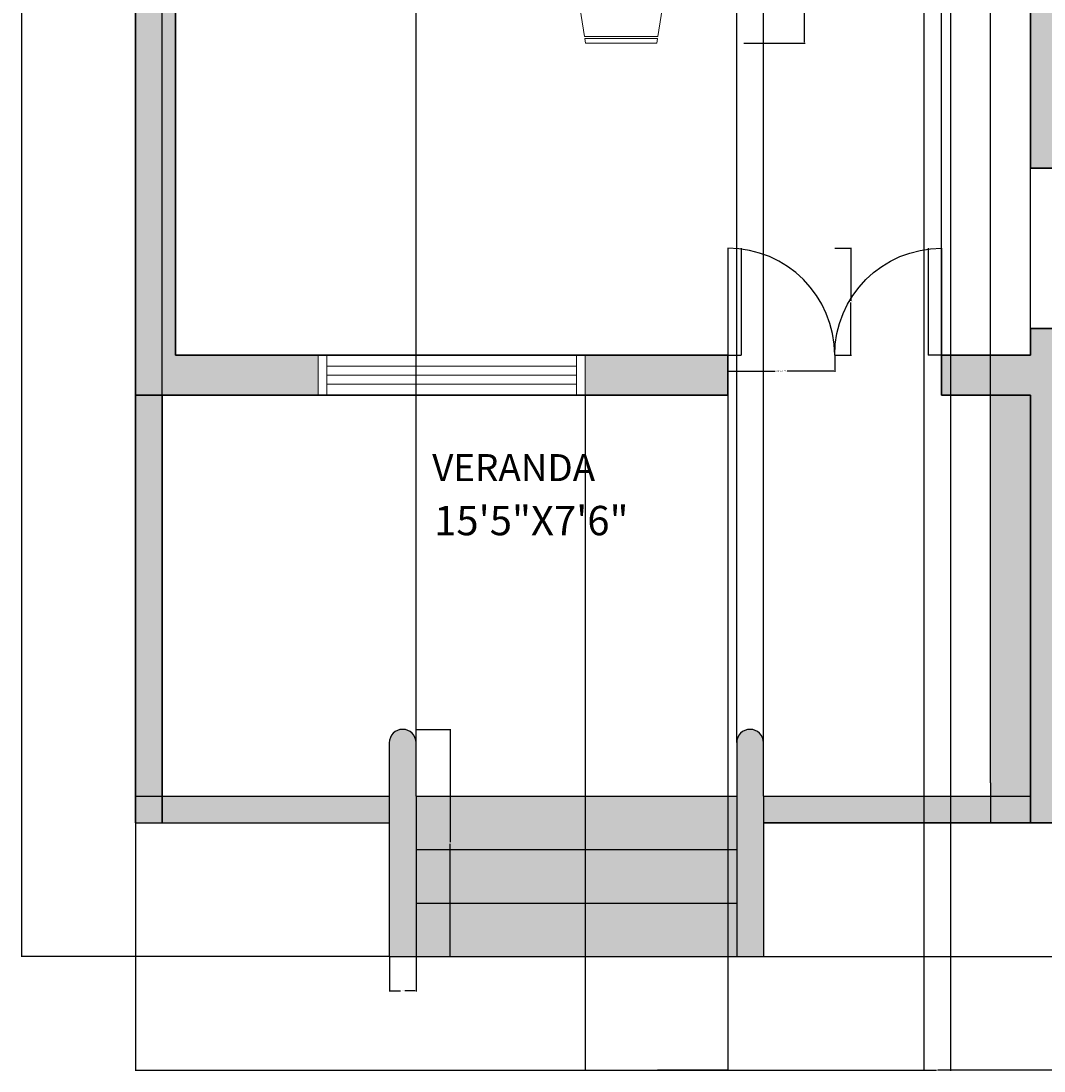
# Model space of a CAD drawing. Units: inches. Extents: x -82 to 330, y 553 to 1115.
# Tile 1 of 4: x -82 to 148, y 553 to 789. Entities that reach past the tile are written whole.
import ezdxf

# ---------------------------------------------------------------- set-up
doc = ezdxf.new("R2010")
doc.units = ezdxf.units.IN
for name, color, linetype, lineweight in [('A-ANNO-DIMS', 2, 'Continuous', 18), ('A-AREA-IDEN', 7, 'Continuous', 25), ('A-DOOR', 3, 'Continuous', 25), ('A-FLOR', 7, 'Continuous', 25), ('A-FLOR-STRS', 7, 'Continuous', 25), ('A-FURN', 8, 'Continuous', 18), ('A-GLAZ', 4, 'Continuous', 18), ('A-WALL', 7, 'Continuous', 35)]:
    doc.layers.add(name, color=color, linetype=linetype, lineweight=lineweight)
doc.layers.add('A-FLOR-PATT', color=252, linetype='Continuous', lineweight=13, true_color=0x939598)
doc.layers.add('A-WALL-PATT', color=18, linetype='Continuous', lineweight=13, true_color=0x000000)
doc.styles.get("Standard").update_dxf_attribs({"font": 'arial.ttf'})
doc.dimstyles.get("Standard").update_dxf_attribs({"dimtxt": 0.18, "dimasz": 0.18, "dimexe": 0.18, "dimexo": 0.0625, "dimgap": 0.09, "dimtad": 0, "dimtih": 1, "dimtoh": 1, "dimdec": 4, "dimzin": 0, "dimdsep": 46, "dimtxsty": 'Standard', "dimcen": 0.09, "dimadec": 0, "dimazin": 0, "dimtfac": 1, "dimtdec": 4, "dimtofl": 0, "dimtmove": 0, "dimatfit": 3, "dimfxl": 1, "dimtolj": 1, "dimtzin": 0, "dimarcsym": 0})

# ---------------------------------------------------------------- blocks, each defined once
blk = doc.blocks.new('Dining Set - 36 x 72 in.')
for p, q in [((-22.2343, 26.00059), (-23.4847, 17.99762)), ((-22.2304, 26), (-5.7608, 26)), ((-22, 27.5), (-22.1562, 26.50042)), ((-5.8416, 26.5), (-22.1534, 26.5)), ((-22, 27.5), (-6, 27.5)), ((-5.8437, 26.49966), (-6, 27.5)), ((-4.5152, 17.99762), (-5.7655, 25.99926)), ((5.7657, 26.00059), (4.5153, 17.99762)), ((5.7696, 26), (22.2392, 26)), ((6, 27.5), (5.8438, 26.50042)), ((22.1584, 26.5), (5.8466, 26.5)), ((6, 27.5), (22, 27.5)), ((22.1563, 26.49966), (22, 27.5)), ((23.4848, 17.99762), (22.2345, 25.99926)), ((36, 18), (-36, 18)), ((-36, 18), (-36, -18)), ((36, -18), (36, 18)), ((-44.0006, 8.23428), (-35.9976, 9.48474)), ((44.0006, 8.23428), (35.9976, 9.48474)), ((-45.5, 8), (-44.5004, 8.15617)), ((-45.5, 8), (-45.5, -8)), ((-44.5, -8.15843), (-44.5, 8.15338)), ((-44, 8.23041), (-44, -8.23915)), ((44, 8.23041), (44, -8.23915)), ((44.5, -8.15843), (44.5, 8.15338)), ((45.5, 8), (44.5005, 8.15617)), ((45.5, 8), (45.5, -8)), ((-44.4997, -8.15631), (-45.5, -8)), ((-35.9976, -9.48476), (-43.9993, -8.2345)), ((35.9976, -9.48476), (43.9993, -8.2345)), ((44.4997, -8.15631), (45.5, -8)), ((-36, -18), (36, -18)), ((-22.2343, -26.0006), (-23.4847, -17.99762)), ((-4.5152, -17.99762), (-5.7655, -25.99928)), ((5.7657, -26.0006), (4.5153, -17.99762)), ((23.4848, -17.99762), (22.2345, -25.99928)), ((-22.2304, -26), (-5.7608, -26)), ((-22, -27.5), (-22.1562, -26.50044)), ((-5.8416, -26.5), (-22.1534, -26.5)), ((-22, -27.5), (-6, -27.5)), ((-5.8437, -26.49967), (-6, -27.5)), ((5.7696, -26), (22.2392, -26)), ((6, -27.5), (5.8438, -26.50044)), ((22.1584, -26.5), (5.8466, -26.5)), ((6, -27.5), (22, -27.5)), ((22.1563, -26.49967), (22, -27.5))]:
    blk.add_line(p, q)
for points in [[(-36, 15), (-31.1772, 14.97754), (-26.8079, 14.91406), (-22.8538, 14.81543), (-19.276, 14.6875), (-16.0362, 14.53613), (-13.0957, 14.36718), (-10.4159, 14.18652), (-7.9583, 14), (-5.6904, 13.81315), (-3.6035, 13.63021), (-1.6954, 13.45508), (0.0365, 13.29166), (1.5945, 13.14388), (2.9811, 13.01562), (4.1988, 12.9108), (5.25, 12.83333), (6.1393, 12.78613), (6.8802, 12.76823), (7.4883, 12.77767), (7.9792, 12.8125), (8.3685, 12.87077), (8.6719, 12.95052), (8.9049, 13.0498), (9.0833, 13.16666), (9.2205, 13.29899), (9.3216, 13.44401), (9.3895, 13.59879), (9.4271, 13.76041), (9.4373, 13.92594), (9.4232, 14.09245), (9.3875, 14.257), (9.3333, 14.41666), (9.2638, 14.56917), (9.1836, 14.71484), (9.0975, 14.85465), (9.0104, 14.98958), (8.9272, 15.1206), (8.8529, 15.2487), (8.7922, 15.37483), (8.75, 15.5), (8.7305, 15.62467), (8.7344, 15.74739), (8.7617, 15.86621), (8.8125, 15.97916), (8.8867, 16.08431), (8.9844, 16.17968), (9.1055, 16.26334), (9.25, 16.33333), (9.4189, 16.38802), (9.6172, 16.42708), (9.8506, 16.45052), (10.125, 16.45833), (10.4463, 16.45052), (10.8203, 16.42708), (11.2529, 16.38802), (11.75, 16.33333), (12.3184, 16.26318), (12.9694, 16.17838), (13.7151, 16.07991), (14.5677, 15.96875), (15.5395, 15.84586), (16.6426, 15.71224), (17.8893, 15.56884), (19.2917, 15.41666), (20.859, 15.25667), (22.5879, 15.08984), (24.4721, 14.91715), (26.5052, 14.73958), (28.6809, 14.5581), (30.9929, 14.3737), (33.4347, 14.18733), (36, 14)], [(-36, 10), (-28.9766, 10.14274), (-23.1725, 10.20442), (-18.4241, 10.19775), (-14.5677, 10.13541), (-11.4399, 10.03011), (-8.877, 9.89453), (-6.7154, 9.74137), (-4.7917, 9.58333), (-2.9698, 9.43082), (-1.2246, 9.28515), (0.4415, 9.14534), (2.026, 9.01041), (3.5266, 8.87939), (4.9408, 8.7513), (6.266, 8.62516), (7.5, 8.5), (8.6411, 8.37549), (9.6914, 8.2539), (10.6538, 8.13818), (11.5312, 8.03125), (12.3267, 7.93603), (13.043, 7.85547), (13.6831, 7.79248), (14.25, 7.75), (14.7471, 7.7303), (15.1797, 7.73307), (15.5537, 7.75732), (15.875, 7.80208), (16.1494, 7.86637), (16.3828, 7.94922), (16.5811, 8.04964), (16.75, 8.16666), (16.8944, 8.29915), (17.0143, 8.44531), (17.1089, 8.60319), (17.1771, 8.77083), (17.218, 8.94629), (17.2305, 9.1276), (17.2137, 9.31282), (17.1667, 9.5), (17.0895, 9.6875), (16.987, 9.875), (16.8649, 10.0625), (16.7292, 10.25), (16.5856, 10.4375), (16.4401, 10.625), (16.2985, 10.8125), (16.1667, 11), (16.05, 11.18733), (15.9518, 11.3737), (15.8752, 11.5581), (15.8229, 11.73958), (15.798, 11.91715), (15.8034, 12.08984), (15.842, 12.25667), (15.9167, 12.41666), (16.0295, 12.56836), (16.1784, 12.70833), (16.3605, 12.83268), (16.5729, 12.9375), (16.8127, 13.01888), (17.0768, 13.07291), (17.3625, 13.0957), (17.6667, 13.08333), (17.9894, 13.03312), (18.3418, 12.94726), (18.7382, 12.82918), (19.1927, 12.68229), (19.7195, 12.51001), (20.3327, 12.31575), (21.0465, 12.10294), (21.875, 11.875), (22.8357, 11.63354), (23.959, 11.37304), (25.2786, 11.08618), (26.8282, 10.76562), (28.6414, 10.40405), (30.752, 9.99414), (33.1936, 9.52856), (36, 9)], [(-36, 5.5), (-30.7157, 5.3348), (-26.069, 5.20963), (-21.9946, 5.11767), (-18.4271, 5.05208), (-15.3009, 5.00602), (-12.5508, 4.97265), (-10.1112, 4.94515), (-7.9167, 4.91666), (-5.909, 4.88167), (-4.0586, 4.83984), (-2.3429, 4.79215), (-0.7396, 4.73958), (0.7739, 4.6831), (2.22, 4.6237), (3.6213, 4.56233), (5, 4.5), (6.373, 4.43782), (7.7344, 4.3776), (9.0723, 4.32129), (10.375, 4.27083), (11.6309, 4.22819), (12.8281, 4.19531), (13.9551, 4.17415), (15, 4.16666), (15.954, 4.17448), (16.819, 4.19791), (17.6001, 4.23698), (18.3021, 4.29166), (18.9299, 4.36198), (19.4883, 4.44791), (19.9823, 4.54948), (20.4167, 4.66666), (20.7969, 4.79899), (21.1302, 4.94401), (21.4245, 5.09879), (21.6875, 5.26041), (21.9271, 5.42594), (22.1511, 5.59245), (22.3672, 5.757), (22.5834, 5.91666), (22.8065, 6.06868), (23.0404, 6.21093), (23.2879, 6.34147), (23.5521, 6.45833), (23.8358, 6.55957), (24.142, 6.64323), (24.4735, 6.70735), (24.8334, 6.75), (25.2235, 6.76969), (25.642, 6.76692), (26.0858, 6.74267), (26.5521, 6.69791), (27.0379, 6.63362), (27.5404, 6.55078), (28.0565, 6.45036), (28.5834, 6.33333), (29.1242, 6.19987), (29.7071, 6.04687), (30.3661, 5.87044), (31.1354, 5.66666), (32.0493, 5.43164), (33.142, 5.16146), (34.4475, 4.85221), (36, 4.5)], [(-36, -1), (-30.7915, -0.6591), (-26.0195, -0.38216), (-21.6519, -0.16284), (-17.6563, 0.00521), (-14.0005, 0.12833), (-10.6523, 0.21289), (-7.5796, 0.26522), (-4.75, 0.29166), (-2.134, 0.29793), (0.2878, 0.28711), (2.5317, 0.26163), (4.6146, 0.22396), (6.5529, 0.17651), (8.3633, 0.12174), (10.0623, 0.06209), (11.6667, 0), (13.1899, -0.06201), (14.6341, -0.1211), (15.9982, -0.17432), (17.2813, -0.21875), (18.4823, -0.25147), (19.6003, -0.26953), (20.6343, -0.27002), (21.5834, -0.25), (22.4481, -0.20768), (23.2357, -0.14584), (23.9549, -0.06836), (24.6146, 0.02083), (25.2235, 0.11784), (25.7904, 0.21875), (26.3241, 0.31966), (26.8334, 0.41666), (27.3265, 0.50618), (27.8099, 0.58593), (28.2894, 0.65397), (28.7709, 0.70833), (29.2601, 0.74707), (29.763, 0.76823), (30.2855, 0.76985), (30.8334, 0.75), (31.4088, 0.70784), (31.9994, 0.64713), (32.589, 0.57275), (33.1615, 0.48958), (33.7008, 0.4025), (34.1908, 0.3164), (34.6153, 0.23616), (34.9584, 0.16666), (35.2099, 0.11165), (35.3848, 0.07031), (35.504, 0.04069), (35.5886, 0.02083), (35.6594, 0.00879), (35.7377, 0.0026), (35.8442, 0.00032), (36, 0)], [(-36, -6.5), (-27.1843, -6.31267), (-20.084, -6.1263), (-14.469, -5.9419), (-10.1094, -5.76042), (-6.7752, -5.58285), (-4.2363, -5.41016), (-2.2629, -5.24333), (-0.625, -5.08334), (0.8708, -4.93099), (2.2715, -4.78646), (3.5872, -4.64974), (4.8281, -4.52084), (6.0046, -4.39974), (7.127, -4.28646), (8.2053, -4.18099), (9.25, -4.08334), (10.2705, -3.99382), (11.2734, -3.91407), (12.2647, -3.84603), (13.25, -3.79167), (14.2354, -3.75293), (15.2266, -3.73177), (16.2295, -3.73015), (17.25, -3.75), (18.2912, -3.79248), (19.3451, -3.85547), (20.4009, -3.93604), (21.4479, -4.03125), (22.4754, -4.13819), (23.4727, -4.25391), (24.4289, -4.37549), (25.3334, -4.5), (26.1785, -4.62492), (26.9694, -4.74935), (27.7145, -4.87281), (28.4219, -4.99479), (29.1, -5.11483), (29.7572, -5.23242), (30.4016, -5.34709), (31.0417, -5.45834), (31.6837, -5.56437), (32.3262, -5.65821), (32.9658, -5.73153), (33.599, -5.77604), (34.2224, -5.78345), (34.8327, -5.74545), (35.4264, -5.65373), (36, -5.5)], [(-36, -10), (-26.4022, -9.81299), (-18.4675, -9.62891), (-11.9839, -9.45069), (-6.7396, -9.28125), (-2.5226, -9.12354), (0.8789, -8.98047), (3.6769, -8.85498), (6.0833, -8.75), (8.2767, -8.66765), (10.3021, -8.60677), (12.1712, -8.56543), (13.8958, -8.54167), (15.4876, -8.53353), (16.9583, -8.53907), (18.3197, -8.55632), (19.5834, -8.58334), (20.7616, -8.61841), (21.8685, -8.66081), (22.9188, -8.71004), (23.9271, -8.76563), (24.9081, -8.82707), (25.8763, -8.89388), (26.8465, -8.96558), (27.8334, -9.04167), (28.8474, -9.12118), (29.8828, -9.20117), (30.93, -9.27824), (31.9792, -9.34896), (33.0205, -9.40991), (34.0443, -9.45768), (35.0407, -9.48885), (36, -9.5)], [(-36, -14.5), (-30.0881, -14.33513), (-25.0332, -14.21224), (-20.7312, -14.12647), (-17.0781, -14.07292), (-13.97, -14.04671), (-11.3027, -14.04297), (-8.9724, -14.05681), (-6.875, -14.08334), (-4.9224, -14.11833), (-3.0905, -14.16016), (-1.3709, -14.20785), (0.2448, -14.26042), (1.7647, -14.3169), (3.1973, -14.3763), (4.5507, -14.43767), (5.8333, -14.5), (7.0554, -14.5621), (8.235, -14.62175), (9.3922, -14.67652), (10.5469, -14.72396), (11.7192, -14.76164), (12.929, -14.78711), (14.1965, -14.79794), (15.5417, -14.79167), (16.9933, -14.76424), (18.6152, -14.70508), (20.4804, -14.60197), (22.6615, -14.44271), (25.2312, -14.21509), (28.2624, -13.9069), (31.8277, -13.50594), (36, -13)]]:
    blk.add_lwpolyline(points)
blk = doc.blocks.new('WIN-60IN')
for p, q in [((60, 9), (0, 9)), ((0, 9), (0, 0)), ((2, 9), (2, 0)), ((58, 0), (58, 9)), ((60, 0), (60, 9)), ((2, 6.5), (58, 6.5)), ((2, 4.5), (58, 4.5)), ((2, 2.5), (58, 2.5)), ((0, 0), (60, 0))]:
    blk.add_line(p, q)
blk = doc.blocks.new('DOOR-LEAF-24IN')
for p, q in [((0, 24), (0, 0)), ((3, 24), (3, 0)), ((0, 0), (3, 0))]:
    blk.add_line(p, q)
blk.add_arc((0, 0), 24, 0, 90)
blk = doc.blocks.new('STAIR-CHEEK-6IN')
for p, q in [((0, 48), (0, 36)), ((6, 36), (6, 48)), ((0, 36), (0, 30)), ((6, 36), (6, 30)), ((0, 30), (0, 0)), ((6, 30), (6, 0)), ((0, 0), (6, 0))]:
    blk.add_line(p, q)
blk.add_arc((3, 48), 3, 0, 180)
blk = doc.blocks.new('*D17')
at = {"layer": 'A-ANNO-DIMS', "color": 0, "lineweight": -2, "transparency": 16777216}
for p, q in [((76.99, 714.05), (76.99, 710.33)), ((100.99, 714.05), (100.99, 710.33)), ((77.17, 710.51), (87.65, 710.51)), ((100.81, 710.51), (90.32, 710.51))]:
    blk.add_line(p, q, dxfattribs=at)
at = {"layer": 'A-ANNO-DIMS', "color": 0, "transparency": 16777216}
for points in [[(77.17, 710.54), (77.17, 710.48), (76.99, 710.51)], [(100.81, 710.54), (100.81, 710.48), (100.99, 710.51)]]:
    blk.add_solid(points, dxfattribs=at)
at = {"layer": 'Defpoints', "color": 0, "transparency": 16777216}
for p in [(76.99, 714.11), (100.99, 714.11), (100.99, 710.51)]:
    blk.add_point(p, dxfattribs=at)
at = {"layer": 'A-ANNO-DIMS', "color": 0, "transparency": 16777216, "insert": (88.99, 710.51), "char_height": 0.18, "attachment_point": 5}
blk.add_mtext('\\A1;ENTRY LEAF 24 TYP.', dxfattribs=at)
blk = doc.blocks.new('*D18')
at = {"layer": 'A-ANNO-DIMS', "color": 0, "lineweight": -2, "transparency": 16777216}
for p, q in [((101.05, 738.11), (104.77, 738.11)), ((104.59, 737.93), (104.59, 726.29)), ((104.59, 714.29), (104.59, 725.93)), ((101.05, 714.11), (104.77, 714.11))]:
    blk.add_line(p, q, dxfattribs=at)
at = {"layer": 'A-ANNO-DIMS', "color": 0, "transparency": 16777216}
for points in [[(104.56, 737.93), (104.62, 737.93), (104.59, 738.11)], [(104.56, 714.29), (104.62, 714.29), (104.59, 714.11)]]:
    blk.add_solid(points, dxfattribs=at)
at = {"layer": 'Defpoints', "color": 0, "transparency": 16777216}
for p in [(100.99, 738.11), (104.59, 738.11), (100.99, 714.11)]:
    blk.add_point(p, dxfattribs=at)
at = {"layer": 'A-ANNO-DIMS', "color": 0, "transparency": 16777216, "insert": (104.59, 726.11), "char_height": 0.18, "attachment_point": 5}
blk.add_mtext('\\A1;24 TYP.', dxfattribs=at)
blk = doc.blocks.new('*D19')
at = {"layer": 'A-ANNO-DIMS', "color": 0, "lineweight": -2, "transparency": 16777216}
for p, q in [((7.05, 630.11), (14.82, 630.11)), ((14.64, 629.93), (14.64, 604.79)), ((14.64, 579.29), (14.64, 604.43)), ((7.05, 579.11), (14.82, 579.11))]:
    blk.add_line(p, q, dxfattribs=at)
at = {"layer": 'A-ANNO-DIMS', "color": 0, "transparency": 16777216}
for points in [[(14.61, 629.93), (14.67, 629.93), (14.64, 630.11)], [(14.61, 579.29), (14.67, 579.29), (14.64, 579.11)]]:
    blk.add_solid(points, dxfattribs=at)
at = {"layer": 'Defpoints', "color": 0, "transparency": 16777216}
for p in [(6.99, 630.11), (14.64, 630.11), (6.99, 579.11)]:
    blk.add_point(p, dxfattribs=at)
at = {"layer": 'A-ANNO-DIMS', "color": 0, "transparency": 16777216, "insert": (14.64, 604.61), "char_height": 0.18, "attachment_point": 5}
blk.add_mtext('\\A1;CHEEK 51 TYP.', dxfattribs=at)
blk = doc.blocks.new('*D20')
at = {"layer": 'A-ANNO-DIMS', "color": 0, "lineweight": -2, "transparency": 16777216}
for p, q in [((0.99, 579.05), (0.99, 571.28)), ((6.99, 579.05), (6.99, 571.28)), ((1.17, 571.46), (3.53, 571.46)), ((6.81, 571.46), (4.45, 571.46))]:
    blk.add_line(p, q, dxfattribs=at)
at = {"layer": 'A-ANNO-DIMS', "color": 0, "transparency": 16777216}
for points in [[(1.17, 571.49), (1.17, 571.43), (0.99, 571.46)], [(6.81, 571.49), (6.81, 571.43), (6.99, 571.46)]]:
    blk.add_solid(points, dxfattribs=at)
at = {"layer": 'Defpoints', "color": 0, "transparency": 16777216}
for p in [(0.99, 579.11), (6.99, 579.11), (6.99, 571.46)]:
    blk.add_point(p, dxfattribs=at)
at = {"layer": 'A-ANNO-DIMS', "color": 0, "transparency": 16777216, "insert": (3.99, 571.46), "char_height": 0.18, "attachment_point": 5}
blk.add_mtext('\\A1;6 TYP.', dxfattribs=at)
blk = doc.blocks.new('*D27')
at = {"layer": 'A-ANNO-DIMS', "color": 0, "lineweight": -2, "transparency": 16777216}
for p, q in [((80.61, 875.16), (94.38, 875.16)), ((94.2, 874.98), (94.2, 829.85)), ((94.2, 784.34), (94.2, 829.48)), ((80.61, 784.16), (94.38, 784.16))]:
    blk.add_line(p, q, dxfattribs=at)
at = {"layer": 'A-ANNO-DIMS', "color": 0, "transparency": 16777216}
for points in [[(94.17, 874.98), (94.23, 874.98), (94.2, 875.16)], [(94.17, 784.34), (94.23, 784.34), (94.2, 784.16)]]:
    blk.add_solid(points, dxfattribs=at)
at = {"layer": 'Defpoints', "color": 0, "transparency": 16777216}
for p in [(80.55, 875.16), (94.2, 875.16), (80.55, 784.16)]:
    blk.add_point(p, dxfattribs=at)
at = {"layer": 'A-ANNO-DIMS', "color": 0, "transparency": 16777216, "insert": (94.2, 829.66), "char_height": 0.18, "attachment_point": 5}
blk.add_mtext('\\A1;DINING SET 91', dxfattribs=at)
blk = doc.blocks.new('*D31')
at = {"layer": 'A-ANNO-DIMS', "color": 0, "lineweight": -2, "transparency": 16777216}
for p, q in [((-56.01, 609.05), (-56.01, 553.43)), ((303.99, 609.05), (303.99, 553.43)), ((-55.83, 553.61), (123.7, 553.61)), ((303.81, 553.61), (124.28, 553.61))]:
    blk.add_line(p, q, dxfattribs=at)
at = {"layer": 'A-ANNO-DIMS', "color": 0, "transparency": 16777216}
for points in [[(-55.83, 553.64), (-55.83, 553.58), (-56.01, 553.61)], [(303.81, 553.64), (303.81, 553.58), (303.99, 553.61)]]:
    blk.add_solid(points, dxfattribs=at)
at = {"layer": 'Defpoints', "color": 0, "transparency": 16777216}
for p in [(-56.01, 609.11), (303.99, 609.11), (303.99, 553.61)]:
    blk.add_point(p, dxfattribs=at)
at = {"layer": 'A-ANNO-DIMS', "color": 0, "transparency": 16777216, "insert": (123.99, 553.61), "char_height": 0.18, "attachment_point": 5}
blk.add_mtext('\\A1;360', dxfattribs=at)
blk = doc.blocks.new('*D32')
at = {"layer": 'A-ANNO-DIMS', "color": 0, "lineweight": -2, "transparency": 16777216}
for p, q in [((-56.07, 1089.11), (-81.69, 1089.11)), ((-81.51, 1088.93), (-81.51, 834.29)), ((-81.51, 579.29), (-81.51, 833.93)), ((0.93, 579.11), (-81.69, 579.11))]:
    blk.add_line(p, q, dxfattribs=at)
at = {"layer": 'A-ANNO-DIMS', "color": 0, "transparency": 16777216}
for points in [[(-81.54, 1088.93), (-81.48, 1088.93), (-81.51, 1089.11)], [(-81.54, 579.29), (-81.48, 579.29), (-81.51, 579.11)]]:
    blk.add_solid(points, dxfattribs=at)
at = {"layer": 'Defpoints', "color": 0, "transparency": 16777216}
for p in [(-81.51, 1089.11), (-56.01, 1089.11), (0.99, 579.11)]:
    blk.add_point(p, dxfattribs=at)
at = {"layer": 'A-ANNO-DIMS', "color": 0, "transparency": 16777216, "insert": (-81.51, 834.11), "char_height": 0.18, "attachment_point": 5}
blk.add_mtext('\\A1;510', dxfattribs=at)
blk = doc.blocks.new('*D35')
at = {"layer": 'A-ANNO-DIMS', "color": 0, "lineweight": -2, "transparency": 16777216}
for p, q in [((84.99, 627.17), (84.99, 1114.79)), ((135.99, 618.17), (135.99, 1114.79)), ((85.17, 1114.61), (110.29, 1114.61)), ((135.81, 1114.61), (110.69, 1114.61))]:
    blk.add_line(p, q, dxfattribs=at)
at = {"layer": 'A-ANNO-DIMS', "color": 0, "transparency": 16777216}
for points in [[(85.17, 1114.64), (85.17, 1114.58), (84.99, 1114.61)], [(135.81, 1114.64), (135.81, 1114.58), (135.99, 1114.61)]]:
    blk.add_solid(points, dxfattribs=at)
at = {"layer": 'Defpoints', "color": 0, "transparency": 16777216}
for p in [(135.99, 1114.61), (84.99, 627.11), (135.99, 618.11)]:
    blk.add_point(p, dxfattribs=at)
at = {"layer": 'A-ANNO-DIMS', "color": 0, "transparency": 16777216, "insert": (110.49, 1114.61), "char_height": 0.18, "attachment_point": 5}
blk.add_mtext('\\A1;51', dxfattribs=at)
blk = doc.blocks.new('*D36')
at = {"layer": 'A-ANNO-DIMS', "color": 0, "lineweight": -2, "transparency": 16777216}
for p, q in [((6.99, 627.17), (6.99, 1114.79)), ((78.99, 627.17), (78.99, 1114.79)), ((7.17, 1114.61), (42.77, 1114.61)), ((78.81, 1114.61), (43.21, 1114.61))]:
    blk.add_line(p, q, dxfattribs=at)
at = {"layer": 'A-ANNO-DIMS', "color": 0, "transparency": 16777216}
for points in [[(7.17, 1114.64), (7.17, 1114.58), (6.99, 1114.61)], [(78.81, 1114.64), (78.81, 1114.58), (78.99, 1114.61)]]:
    blk.add_solid(points, dxfattribs=at)
at = {"layer": 'Defpoints', "color": 0, "transparency": 16777216}
for p in [(78.99, 1114.61), (6.99, 627.11), (78.99, 627.11)]:
    blk.add_point(p, dxfattribs=at)
at = {"layer": 'A-ANNO-DIMS', "color": 0, "transparency": 16777216, "insert": (42.99, 1114.61), "char_height": 0.18, "attachment_point": 5}
blk.add_mtext('\\A1;72', dxfattribs=at)
blk = doc.blocks.new('*D37')
at = {"layer": 'A-ANNO-DIMS', "color": 0, "lineweight": -2, "transparency": 16777216}
for p, q in [((85.05, 609.11), (329.67, 609.11)), ((329.49, 608.93), (329.49, 594.29)), ((329.49, 579.29), (329.49, 593.93)), ((85.05, 579.11), (329.67, 579.11))]:
    blk.add_line(p, q, dxfattribs=at)
at = {"layer": 'A-ANNO-DIMS', "color": 0, "transparency": 16777216}
for points in [[(329.46, 608.93), (329.52, 608.93), (329.49, 609.11)], [(329.46, 579.29), (329.52, 579.29), (329.49, 579.11)]]:
    blk.add_solid(points, dxfattribs=at)
at = {"layer": 'Defpoints', "color": 0, "transparency": 16777216}
for p in [(84.99, 609.11), (329.49, 609.11), (84.99, 579.11)]:
    blk.add_point(p, dxfattribs=at)
at = {"layer": 'A-ANNO-DIMS', "color": 0, "transparency": 16777216, "insert": (329.49, 594.11), "char_height": 0.18, "attachment_point": 5}
blk.add_mtext('\\A1;30', dxfattribs=at)
blk = doc.blocks.new('*D41')
at = {"layer": 'A-ANNO-DIMS', "color": 0, "lineweight": -2, "transparency": 16777216}
for p, q in [((124.99, 714.17), (124.99, 1114.79)), ((144.99, 714.17), (144.99, 1114.79)), ((125.17, 1114.61), (134.77, 1114.61)), ((144.81, 1114.61), (135.21, 1114.61))]:
    blk.add_line(p, q, dxfattribs=at)
at = {"layer": 'A-ANNO-DIMS', "color": 0, "transparency": 16777216}
for points in [[(125.17, 1114.64), (125.17, 1114.58), (124.99, 1114.61)], [(144.81, 1114.64), (144.81, 1114.58), (144.99, 1114.61)]]:
    blk.add_solid(points, dxfattribs=at)
at = {"layer": 'Defpoints', "color": 0, "transparency": 16777216}
for p in [(144.99, 1114.61), (124.99, 714.11), (144.99, 714.11)]:
    blk.add_point(p, dxfattribs=at)
at = {"layer": 'A-ANNO-DIMS', "color": 0, "transparency": 16777216, "insert": (134.99, 1114.61), "char_height": 0.18, "attachment_point": 5}
blk.add_mtext('\\A1;20', dxfattribs=at)
blk = doc.blocks.new('*D42')
at = {"layer": 'A-ANNO-DIMS', "color": 0, "lineweight": -2, "transparency": 16777216}
for p, q in [((44.99, 705.05), (44.99, 553.43)), ((76.99, 705.05), (76.99, 553.43)), ((45.17, 553.61), (60.77, 553.61)), ((76.81, 553.61), (61.21, 553.61))]:
    blk.add_line(p, q, dxfattribs=at)
at = {"layer": 'A-ANNO-DIMS', "color": 0, "transparency": 16777216}
for points in [[(45.17, 553.64), (45.17, 553.58), (44.99, 553.61)], [(76.81, 553.64), (76.81, 553.58), (76.99, 553.61)]]:
    blk.add_solid(points, dxfattribs=at)
at = {"layer": 'Defpoints', "color": 0, "transparency": 16777216}
for p in [(44.99, 705.11), (76.99, 705.11), (76.99, 553.61)]:
    blk.add_point(p, dxfattribs=at)
at = {"layer": 'A-ANNO-DIMS', "color": 0, "transparency": 16777216, "insert": (60.99, 553.61), "char_height": 0.18, "attachment_point": 5}
blk.add_mtext('\\A1;32', dxfattribs=at)
blk = doc.blocks.new('*D43')
at = {"layer": 'A-ANNO-DIMS', "color": 0, "lineweight": -2, "transparency": 16777216}
for p, q in [((120.99, 1080.05), (120.99, 553.43)), ((126.99, 1080.05), (126.99, 553.43)), ((121.17, 553.61), (123.84, 553.61)), ((126.81, 553.61), (124.14, 553.61))]:
    blk.add_line(p, q, dxfattribs=at)
at = {"layer": 'A-ANNO-DIMS', "color": 0, "transparency": 16777216}
for points in [[(121.17, 553.64), (121.17, 553.58), (120.99, 553.61)], [(126.81, 553.64), (126.81, 553.58), (126.99, 553.61)]]:
    blk.add_solid(points, dxfattribs=at)
at = {"layer": 'Defpoints', "color": 0, "transparency": 16777216}
for p in [(120.99, 1080.11), (126.99, 1080.11), (126.99, 553.61)]:
    blk.add_point(p, dxfattribs=at)
at = {"layer": 'A-ANNO-DIMS', "color": 0, "transparency": 16777216, "insert": (123.99, 553.61), "char_height": 0.18, "attachment_point": 5}
blk.add_mtext('\\A1;6', dxfattribs=at)
blk = doc.blocks.new('*D48')
at = {"layer": 'A-ANNO-DIMS', "color": 0, "lineweight": -2, "transparency": 16777216}
for p, q in [((-50.01, 609.17), (-50.01, 1114.79)), ((135.99, 618.17), (135.99, 1114.79)), ((-49.83, 1114.61), (42.71, 1114.61)), ((135.81, 1114.61), (43.27, 1114.61))]:
    blk.add_line(p, q, dxfattribs=at)
at = {"layer": 'A-ANNO-DIMS', "color": 0, "transparency": 16777216}
for points in [[(-49.83, 1114.64), (-49.83, 1114.58), (-50.01, 1114.61)], [(135.81, 1114.64), (135.81, 1114.58), (135.99, 1114.61)]]:
    blk.add_solid(points, dxfattribs=at)
at = {"layer": 'Defpoints', "color": 0, "transparency": 16777216}
for p in [(135.99, 1114.61), (135.99, 618.11), (-50.01, 609.11)]:
    blk.add_point(p, dxfattribs=at)
at = {"layer": 'A-ANNO-DIMS', "color": 0, "transparency": 16777216, "insert": (42.99, 1114.61), "char_height": 0.18, "attachment_point": 5}
blk.add_mtext('\\A1;186', dxfattribs=at)

msp = doc.modelspace()

# ---------------------------------------------------------------- hatches: boundary and pattern name
at = {"layer": 'A-FLOR-PATT'}
h = msp.add_hatch(color=256, dxfattribs=at)
h.dxf.hatch_style = 1
h.paths.add_polyline_path([(-50.012, 705.11), (-56.012, 705.11), (-56.012, 615.11), (-50.012, 615.11)])
h.paths.add_polyline_path([(0.988, 615.11), (-50.012, 615.11), (-50.012, 609.11), (0.988, 609.11)])
h.paths.add_polyline_path([(6.988, 627.11, 1), (0.988, 627.11), (0.988, 615.11), (0.988, 609.11), (0.988, 579.11), (6.988, 579.11), (6.988, 609.11), (6.988, 615.11)])
h.paths.add_polyline_path([(78.988, 609.11), (78.988, 615.11), (6.988, 615.11), (6.988, 609.11), (6.988, 603.11), (78.988, 603.11)])
h.paths.add_polyline_path([(78.988, 603.11), (6.988, 603.11), (6.988, 591.11), (78.988, 591.11)])
h.paths.add_polyline_path([(135.988, 615.11), (84.988, 615.11), (84.988, 609.11), (135.988, 609.11)])
h.paths.add_polyline_path([(144.988, 705.11), (135.988, 705.11), (135.988, 618.11), (135.988, 615.11), (144.988, 615.11), (144.988, 618.11)])
h.paths.add_polyline_path([(78.988, 591.11), (6.988, 591.11), (6.988, 579.11), (78.988, 579.11)])
h.paths.add_polyline_path([(84.988, 615.11), (84.988, 627.11, 1), (78.988, 627.11), (78.988, 615.11), (78.988, 609.11), (78.988, 603.11), (78.988, 579.11), (84.988, 579.11), (84.988, 609.11)])
at = {"layer": 'A-WALL-PATT'}
h = msp.add_hatch(color=256, dxfattribs=at)
h.dxf.hatch_style = 1
h.paths.add_polyline_path([(6.988, 1089.11), (-56.012, 1089.11), (-56.012, 705.11), (-47.012, 705.11), (-15.012, 705.11), (-15.012, 714.11), (-47.012, 714.11), (-47.012, 930.11), (79.988, 930.11), (79.988, 936.11), (-47.012, 936.11), (-47.012, 1080.11), (6.988, 1080.11)])
h.paths.add_polyline_path([(180.988, 1089.11), (66.988, 1089.11), (66.988, 1080.11), (120.988, 1080.11), (120.988, 936.11), (115.988, 936.11), (115.988, 930.11), (131.988, 930.11), (131.988, 936.11), (126.988, 936.11), (126.988, 1080.11), (180.988, 1080.11)])
h.paths.add_polyline_path([(303.988, 1089.11), (240.988, 1089.11), (240.988, 1080.11), (294.988, 1080.11), (294.988, 936.11), (167.988, 936.11), (167.988, 930.11), (180.988, 930.11), (180.988, 834.11), (186.988, 834.11), (186.988, 930.11), (294.988, 930.11), (294.988, 867.11), (303.988, 867.11)])
h.paths.add_polyline_path([(303.988, 855.11), (294.988, 855.11), (294.988, 792.11), (186.988, 792.11), (186.988, 804.11), (180.988, 804.11), (180.988, 792.11), (144.988, 792.11), (144.988, 756.11), (150.988, 756.11), (150.988, 786.11), (294.988, 786.11), (294.988, 732.11), (303.988, 732.11)])
h.paths.add_polyline_path([(303.988, 672.11), (294.988, 672.11), (294.988, 618.11), (150.988, 618.11), (150.988, 720.11), (144.988, 720.11), (144.988, 714.11), (124.988, 714.11), (124.988, 705.11), (144.988, 705.11), (144.988, 618.11), (144.988, 609.11), (303.988, 609.11)])
h.paths.add_polyline_path([(76.988, 714.11), (44.988, 714.11), (44.988, 705.11), (76.988, 705.11)], flags=17)
h = msp.add_hatch(color=256, dxfattribs=at)
h.dxf.hatch_style = 1
h.paths.add_polyline_path([(-50.012, 615.11), (-56.012, 615.11), (-56.012, 609.11), (-50.012, 609.11)])
h.paths.add_polyline_path([(144.988, 615.11), (135.988, 615.11), (135.988, 609.11), (144.988, 609.11)])
h.paths.add_polyline_path([(-47.012, 930.11), (79.988, 930.11), (79.988, 936.11), (-47.012, 936.11), (-47.012, 1080.11), (6.988, 1080.11), (6.988, 1089.11), (-56.012, 1089.11), (-56.012, 705.11), (-47.012, 705.11), (-15.012, 705.11), (-15.012, 714.11), (-47.012, 714.11)])

# ---------------------------------------------------------------- linework, layer by layer
at = {"layer": 'A-FLOR'}
for p, q in [((-50.012, 705.11), (-50.012, 609.11)), ((135.988, 618.11), (135.988, 705.11)), ((135.988, 618.11), (135.988, 609.11)), ((-56.012, 615.11), (0.988, 615.11)), ((84.988, 615.11), (144.988, 615.11)), ((-56.012, 609.11), (0.988, 609.11))]:
    msp.add_line(p, q, dxfattribs=at)
at = {"layer": 'A-FLOR-STRS'}
for p, q in [((6.988, 615.11), (78.988, 615.11)), ((6.988, 603.11), (78.988, 603.11)), ((6.988, 591.11), (78.988, 591.11)), ((6.988, 579.11), (78.988, 579.11))]:
    msp.add_line(p, q, dxfattribs=at)
at = {"layer": 'A-WALL'}
for p, q in [((-56.012, 1089.11), (-56.012, 609.11)), ((-47.012, 930.11), (-47.012, 714.11)), ((144.988, 756.11), (144.988, 792.11)), ((150.988, 756.11), (144.988, 756.11)), ((150.988, 720.11), (144.988, 720.11)), ((144.988, 714.11), (144.988, 720.11)), ((76.988, 714.11), (-47.012, 714.11)), ((76.988, 714.11), (76.988, 705.11)), ((144.988, 714.11), (124.988, 714.11)), ((124.988, 714.11), (124.988, 705.11)), ((-47.012, 705.11), (-56.012, 705.11)), ((76.988, 705.11), (-47.012, 705.11)), ((144.988, 705.11), (124.988, 705.11)), ((144.988, 618.11), (144.988, 705.11)), ((144.988, 618.11), (144.988, 609.11)), ((84.988, 609.11), (303.988, 609.11))]:
    msp.add_line(p, q, dxfattribs=at)

# ---------------------------------------------------------------- block references
at = {"layer": 'A-DOOR'}
msp.add_blockref('DOOR-LEAF-24IN', (76.988, 714.11), dxfattribs=at)
at = {"layer": 'A-DOOR', "extrusion": (0, 0, -1), "zscale": -1}
msp.add_blockref('DOOR-LEAF-24IN', (-124.989, 714.11), dxfattribs=at)
at = {"layer": 'A-FLOR-STRS'}
for p in [(0.988, 579.11), (78.988, 579.11)]:
    msp.add_blockref('STAIR-CHEEK-6IN', p, dxfattribs=at)
at = {"layer": 'A-FURN', "rotation": 90}
msp.add_blockref('Dining Set - 36 x 72 in.', (53.047, 829.664), dxfattribs=at)
at = {"layer": 'A-GLAZ'}
msp.add_blockref('WIN-60IN', (-15.012, 705.11), dxfattribs=at)

# ---------------------------------------------------------------- texts
at = {"layer": 'A-AREA-IDEN', "attachment_point": 1}
for s, width, gutter_width, insert, char_height in [('VERANDA', 272.11251, 30.289, (10.618, 691.896), 6.0578), ('15\'5"X7\'6"', 296.19152, 32.969, (11.051, 680.274), 6.5939)]:
    msp.add_mtext_dynamic_manual_height_columns(s, width=width, gutter_width=gutter_width, heights=[0], dxfattribs=dict(at, insert=insert, char_height=char_height))

# ---------------------------------------------------------------- dimensions: what is measured, and where the dimension line sits
at = {"layer": 'A-ANNO-DIMS'}
for base, p1, p2, picture, middle in [((135.988, 1114.611), (-50.012, 609.11), (135.988, 618.11), '*D48', (42.988, 1114.611)), ((78.988, 1114.611), (6.988, 627.11), (78.988, 627.11), '*D36', (42.988, 1114.611)), ((135.988, 1114.611), (84.988, 627.11), (135.988, 618.11), '*D35', (110.488, 1114.611)), ((144.988, 1114.611), (124.988, 714.11), (144.988, 714.11), '*D41', (134.988, 1114.611)), ((126.988, 553.609), (120.988, 1080.11), (126.988, 1080.11), '*D43', (123.988, 553.609)), ((76.988, 553.609), (44.988, 705.11), (76.988, 705.11), '*D42', (60.988, 553.609)), ((303.988, 553.609), (-56.012, 609.11), (303.988, 609.11), '*D31', (123.988, 553.609))]:
    dim = msp.add_linear_dim(base=base, p1=p1, p2=p2, dimstyle='Standard', override={"dimdec": 0, "dimlfac": 1, "dimrnd": 0, "dimzin": 0, "dimdsep": 46, "dimlunit": 2}, dxfattribs=at)
    dim.commit()
    dim.dimension.update_dxf_attribs({"geometry": picture, "text_midpoint": middle})
for base, p1, p2, picture, middle in [((-81.513, 1089.11), (0.988, 579.11), (-56.012, 1089.11), '*D32', (-81.513, 834.11)), ((329.489, 609.11), (84.988, 579.11), (84.988, 609.11), '*D37', (329.489, 594.11))]:
    dim = msp.add_linear_dim(base=base, p1=p1, p2=p2, angle=90, dimstyle='Standard', override={"dimdec": 0, "dimlfac": 1, "dimrnd": 0, "dimzin": 0, "dimdsep": 46, "dimlunit": 2}, dxfattribs=at)
    dim.commit()
    dim.dimension.update_dxf_attribs({"geometry": picture, "text_midpoint": middle})
for base, p1, p2, text, picture, middle in [((94.197, 875.164), (80.547, 784.164), (80.547, 875.164), 'DINING SET <>', '*D27', (94.197, 829.664)), ((104.588, 738.11), (100.988, 714.11), (100.988, 738.11), '<> TYP.', '*D18', (104.588, 726.11)), ((14.638, 630.11), (6.988, 579.11), (6.988, 630.11), 'CHEEK <> TYP.', '*D19', (14.638, 604.61))]:
    dim = msp.add_linear_dim(base=base, p1=p1, p2=p2, angle=90, text=text, dimstyle='Standard', override={"dimdec": 0, "dimlfac": 1, "dimrnd": 0, "dimzin": 0, "dimdsep": 46, "dimlunit": 2}, dxfattribs=at)
    dim.commit()
    dim.dimension.update_dxf_attribs({"geometry": picture, "text_midpoint": middle})
for base, p1, p2, text, picture, middle in [((100.988, 710.51), (76.988, 714.11), (100.988, 714.11), 'ENTRY LEAF <> TYP.', '*D17', (88.988, 710.51)), ((6.988, 571.46), (0.988, 579.11), (6.988, 579.11), '<> TYP.', '*D20', (3.988, 571.46))]:
    dim = msp.add_linear_dim(base=base, p1=p1, p2=p2, text=text, dimstyle='Standard', override={"dimdec": 0, "dimlfac": 1, "dimrnd": 0, "dimzin": 0, "dimdsep": 46, "dimlunit": 2}, dxfattribs=at)
    dim.commit()
    dim.dimension.update_dxf_attribs({"geometry": picture, "text_midpoint": middle})

doc.saveas('drawing.dxf')
